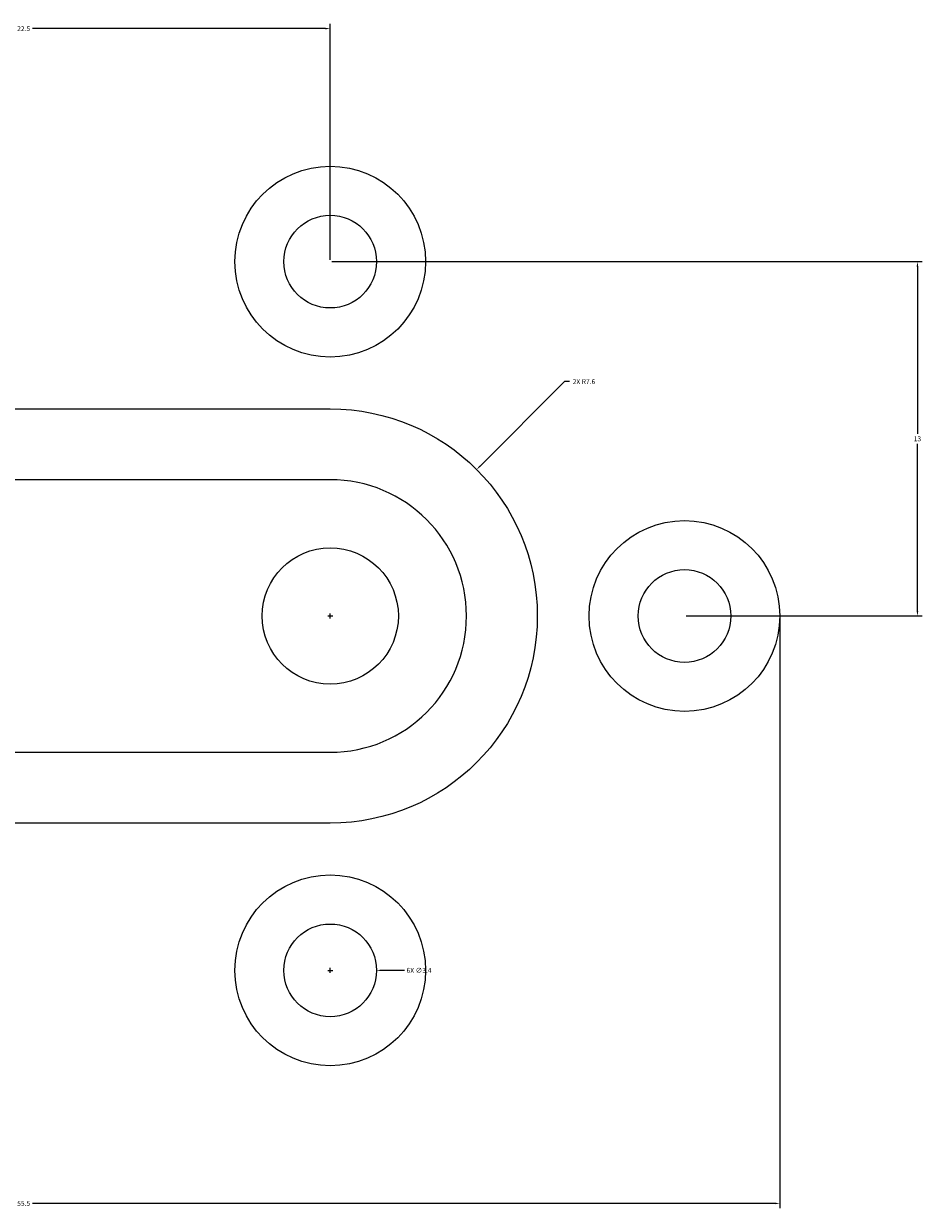
# Model space of a CAD drawing. Units: millimetres. Extents: x 3243.8 to 3309.8, y 1625.7 to 1669.2.
# Tile 3 of 3: x 3276.8 to 3309.8, y 1625.7 to 1669.2. Entities that reach past the tile are written whole.
import ezdxf

# ---------------------------------------------------------------- set-up
doc = ezdxf.new("R2010")
doc.units = ezdxf.units.MM
doc.layers.add('M-CONS', color=8, linetype='Continuous', lineweight=18)
doc.layers.add('M-DIMS', color=2, linetype='Continuous', lineweight=18)
doc.styles.get("Standard").update_dxf_attribs({"font": 'arial.ttf'})
doc.dimstyles.get("Standard").update_dxf_attribs({"dimtxt": 0.18, "dimasz": 0.18, "dimexe": 0.18, "dimexo": 0.0625, "dimgap": 0.09, "dimtad": 0, "dimtih": 1, "dimtoh": 1, "dimdec": 4, "dimzin": 0, "dimdsep": 46, "dimtxsty": 'Standard', "dimcen": 0.09, "dimadec": 0, "dimazin": 0, "dimtfac": 1, "dimtdec": 4, "dimtofl": 0, "dimtmove": 0, "dimatfit": 3, "dimfxl": 1, "dimtolj": 1, "dimtzin": 0, "dimarcsym": 0})

# ---------------------------------------------------------------- blocks, each defined once
blk = doc.blocks.new('CBORE-7-BORE-3.4')
for centre, radius in [((3.5, 3.5), 3.5), ((3.5, 3.5, -1), 1.7)]:
    blk.add_circle(centre, radius)
blk = doc.blocks.new('*D2')
at = {"layer": 'Defpoints', "color": 0, "transparency": 16777216}
for p in [(3249.045, 1647.47), (3304.545, 1647.47), (3304.545, 1625.92)]:
    blk.add_point(p, dxfattribs=at)
at = {"layer": 'M-DIMS', "color": 0, "lineweight": -2, "transparency": 16777216}
for p, q in [((3249.045, 1647.407), (3249.045, 1625.74)), ((3304.545, 1647.407), (3304.545, 1625.74)), ((3249.225, 1625.92), (3276.47, 1625.92)), ((3304.365, 1625.92), (3277.119, 1625.92))]:
    blk.add_line(p, q, dxfattribs=at)
at = {"layer": 'M-DIMS', "color": 0, "transparency": 16777216}
for points in [[(3249.225, 1625.95), (3249.225, 1625.89), (3249.045, 1625.92)], [(3304.365, 1625.95), (3304.365, 1625.89), (3304.545, 1625.92)]]:
    blk.add_solid(points, dxfattribs=at)
at = {"layer": 'M-DIMS', "color": 0, "transparency": 16777216, "insert": (3276.795, 1625.92), "char_height": 0.18, "attachment_point": 5}
blk.add_mtext('\\A1;55.5', dxfattribs=at)
blk = doc.blocks.new('*D5')
at = {"layer": 'Defpoints', "color": 0, "transparency": 16777216}
for p in [(3288.045, 1669.02), (3265.545, 1660.47), (3288.045, 1660.47)]:
    blk.add_point(p, dxfattribs=at)
at = {"layer": 'M-DIMS', "color": 0, "lineweight": -2, "transparency": 16777216}
for p, q in [((3265.545, 1660.532), (3265.545, 1669.2)), ((3265.725, 1669.02), (3276.469, 1669.02)), ((3287.865, 1669.02), (3277.121, 1669.02)), ((3288.045, 1660.532), (3288.045, 1669.2))]:
    blk.add_line(p, q, dxfattribs=at)
at = {"layer": 'M-DIMS', "color": 0, "transparency": 16777216}
for points in [[(3265.725, 1669.05), (3265.725, 1668.99), (3265.545, 1669.02)], [(3287.865, 1669.05), (3287.865, 1668.99), (3288.045, 1669.02)]]:
    blk.add_solid(points, dxfattribs=at)
at = {"layer": 'M-DIMS', "color": 0, "transparency": 16777216, "insert": (3276.795, 1669.02), "char_height": 0.18, "attachment_point": 5}
blk.add_mtext('\\A1;22.5', dxfattribs=at)
blk = doc.blocks.new('*D6')
at = {"layer": 'Defpoints', "color": 0, "transparency": 16777216}
for p in [(3288.045, 1660.47), (3309.595, 1660.47), (3301.045, 1647.47)]:
    blk.add_point(p, dxfattribs=at)
at = {"layer": 'M-DIMS', "color": 0, "lineweight": -2, "transparency": 16777216}
for p, q in [((3288.107, 1660.47), (3309.775, 1660.47)), ((3309.595, 1660.29), (3309.595, 1654.152)), ((3309.595, 1647.65), (3309.595, 1653.788)), ((3301.107, 1647.47), (3309.775, 1647.47))]:
    blk.add_line(p, q, dxfattribs=at)
at = {"layer": 'M-DIMS', "color": 0, "transparency": 16777216}
for points in [[(3309.565, 1660.29), (3309.625, 1660.29), (3309.595, 1660.47)], [(3309.565, 1647.65), (3309.625, 1647.65), (3309.595, 1647.47)]]:
    blk.add_solid(points, dxfattribs=at)
at = {"layer": 'M-DIMS', "color": 0, "transparency": 16777216, "insert": (3309.595, 1653.97), "char_height": 0.18, "attachment_point": 5}
blk.add_mtext('\\A1;13', dxfattribs=at)
blk = doc.blocks.new('*D7')
at = {"layer": 'Defpoints', "color": 0, "transparency": 16777216}
for p in [(3293.419, 1652.844), (3288.045, 1647.47)]:
    blk.add_point(p, dxfattribs=at)
at = {"layer": 'M-DIMS', "color": 0, "lineweight": -2, "transparency": 16777216}
for p, q in [((3296.643, 1656.068), (3293.546, 1652.971)), ((3296.823, 1656.068), (3296.643, 1656.068)), ((3287.955, 1647.47), (3288.135, 1647.47)), ((3288.045, 1647.38), (3288.045, 1647.56))]:
    blk.add_line(p, q, dxfattribs=at)
at = {"layer": 'M-DIMS', "color": 0, "transparency": 16777216}
blk.add_solid([(3293.525, 1652.992), (3293.567, 1652.95), (3293.419, 1652.844)], dxfattribs=at)
at = {"layer": 'M-DIMS', "color": 0, "transparency": 16777216, "insert": (3297.358, 1656.068), "char_height": 0.18, "attachment_point": 5}
blk.add_mtext('\\A1;2X R7.6', dxfattribs=at)
blk = doc.blocks.new('*D10')
at = {"layer": 'Defpoints', "color": 0, "transparency": 16777216}
for p in [(3286.345, 1634.47), (3289.745, 1634.47)]:
    blk.add_point(p, dxfattribs=at)
at = {"layer": 'M-DIMS', "color": 0, "lineweight": -2, "transparency": 16777216}
for p, q in [((3288.045, 1634.38), (3288.045, 1634.56)), ((3287.955, 1634.47), (3288.135, 1634.47)), ((3290.765, 1634.47), (3289.925, 1634.47))]:
    blk.add_line(p, q, dxfattribs=at)
at = {"layer": 'M-DIMS', "color": 0, "transparency": 16777216}
blk.add_solid([(3289.925, 1634.5), (3289.925, 1634.44), (3289.745, 1634.47)], dxfattribs=at)
at = {"layer": 'M-DIMS', "color": 0, "transparency": 16777216, "insert": (3291.305, 1634.47), "char_height": 0.18, "attachment_point": 5}
blk.add_mtext('\\A1;6X ∅3.4', dxfattribs=at)

msp = doc.modelspace()

# ---------------------------------------------------------------- linework, layer by layer
at = {"layer": 'M-CONS'}
for points in [[(3265.545, 1655.07), (3288.045, 1655.07, -1), (3288.045, 1639.87), (3265.545, 1639.87, -1)], [(3288.045, 1652.47), (3265.545, 1652.47, 1), (3265.545, 1642.47), (3288.045, 1642.47, 1)]]:
    msp.add_lwpolyline(points, format="xyb", close=True, dxfattribs=at)
for centre, radius in [((3288.045, 1660.47), 3.5), ((3288.045, 1660.47, -1), 1.7), ((3301.045, 1647.47), 3.5), ((3288.045, 1647.47), 2.5), ((3288.045, 1634.47), 3.5)]:
    msp.add_circle(centre, radius, dxfattribs=at)

# ---------------------------------------------------------------- block references
for p in [(3284.545, 1656.97), (3297.545, 1643.97), (3284.545, 1630.97)]:
    msp.add_blockref('CBORE-7-BORE-3.4', p, dxfattribs=at)

# ---------------------------------------------------------------- dimensions: what is measured, and where the dimension line sits
at = {"layer": 'M-DIMS'}
for base, p1, p2, picture, middle in [((3288.045, 1669.02), (3265.545, 1660.47), (3288.045, 1660.47), '*D5', (3276.795, 1669.02)), ((3304.545, 1625.92), (3249.045, 1647.47), (3304.545, 1647.47), '*D2', (3276.795, 1625.92))]:
    dim = msp.add_linear_dim(base=base, p1=p1, p2=p2, dimstyle='Standard', override={"dimdec": 1, "dimlfac": 1, "dimrnd": 0, "dimzin": 0, "dimdsep": 46, "dimlunit": 2}, dxfattribs=at)
    dim.commit()
    dim.dimension.update_dxf_attribs({"geometry": picture, "text_midpoint": middle})
dim = msp.add_linear_dim(base=(3309.595, 1660.47), p1=(3301.045, 1647.47), p2=(3288.045, 1660.47), angle=90, dimstyle='Standard', override={"dimdec": 0, "dimlfac": 1, "dimrnd": 0, "dimzin": 0, "dimdsep": 46, "dimlunit": 2}, dxfattribs=at)
dim.commit()
dim.dimension.update_dxf_attribs({"geometry": '*D6', "text_midpoint": (3309.595, 1653.97)})
dim = msp.add_radius_dim(center=(3288.045, 1647.47), mpoint=(3293.419, 1652.844), text='2X <>', dimstyle='Standard', override={"dimdec": 1, "dimlfac": 1, "dimrnd": 0, "dimzin": 0, "dimdsep": 46, "dimlunit": 2}, dxfattribs=at)
dim.commit()
dim.dimension.update_dxf_attribs({"geometry": '*D7', "text_midpoint": (3297.358, 1656.068), "dimtype": 164})
dim = msp.add_diameter_dim_2p(p1=(3286.345, 1634.47), p2=(3289.745, 1634.47), text='6X <>', dimstyle='Standard', override={"dimdec": 1, "dimlfac": 1, "dimrnd": 0, "dimzin": 0, "dimdsep": 46, "dimlunit": 2}, dxfattribs=at)
dim.commit()
dim.dimension.update_dxf_attribs({"geometry": '*D10', "text_midpoint": (3290.765, 1634.47), "dimtype": 163})

doc.saveas('drawing.dxf')
